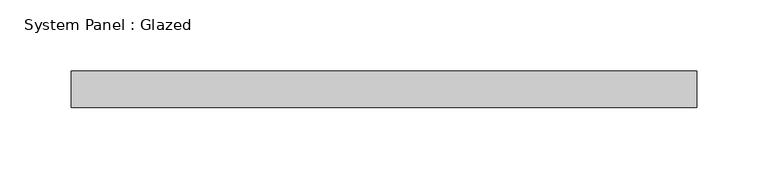
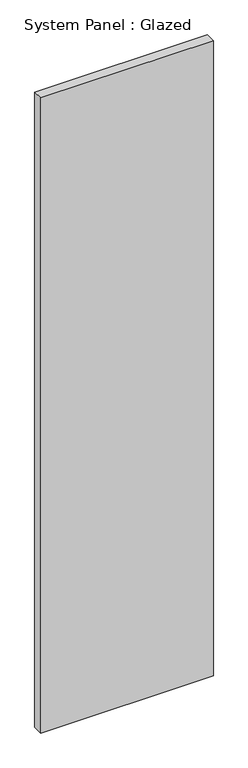
"""IFC4 building model written with IfcOpenShell, lengths in millimetres: plate geometry, System Panel : Glazed."""

from ifc_helpers import new_model, si_unit, origin, origin_with_axes, place, context, project, spatial, polyline, outline, extrude, source, transform, mapped, element, save


def system_panel_glazed_a5d4ee92(model_context):
    return source(origin(), model_context, "Body", "SweptSolid", [
        extrude(outline(polyline([(219.075, 19.05), (-219.075, 19.05), (-219.075, 44.45), (219.075, 44.45), (219.075, 19.05)])), origin_with_axes(), (0.0, 0.0, 1.0), 1701.8),
    ])


if __name__ == "__main__":
    model = new_model("IFC4")
    model_context = context("Model", 3, world=origin())
    ifc_project = project(units=[si_unit("LENGTHUNIT", "METRE", prefix="MILLI")], contexts=[model_context])
    site = spatial("IfcSite", under=ifc_project)
    building = spatial("IfcBuilding", under=site)
    placement = place(None, origin())
    system_panel_glazed_shape = system_panel_glazed_a5d4ee92(model_context)
    element("IfcPlate", 1, ObjectType="System Panel : Glazed", at=placement, inside=building, context=model_context, shape_type="MappedRepresentation", body=[
        mapped(system_panel_glazed_shape, transform((0.0, 0.0, 0.0), x_axis=(1.0, 0.0, 0.0), y_axis=(0.0, 1.0, 0.0), z_axis=(0.0, 0.0, 1.0))),
    ])
    save(model, "model.ifc")

# Revit data of these elements
# Type "System Panel : Glazed"
#   Construction Type Id = "GSP4R"
#   Analytic Construction = "1/8 in Pilkington single glazing"
#   Visual Light Transmittance = 0.9
#   Solar Heat Gain Coefficient = 0.86
#   Heat Transfer Coefficient (U) = 1.18115 BTU/(h·ft²·°F)
#   Define Thermal Properties by = 1
# Element 1 (IfcPlate, "System Panel : Glazed")
#   Materials on its faces: "Glass"
# Materials
#   "Glass": class "Glass", colour RGB 0 128 192, transparency 0.75, Description = "Soda Lime Glass", Cost = 0
